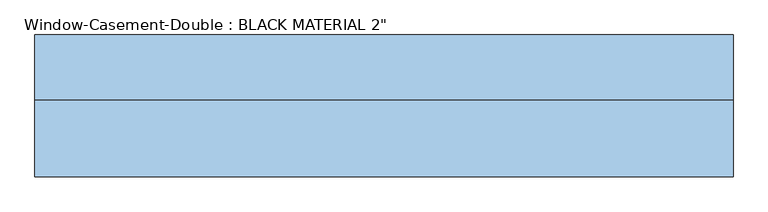
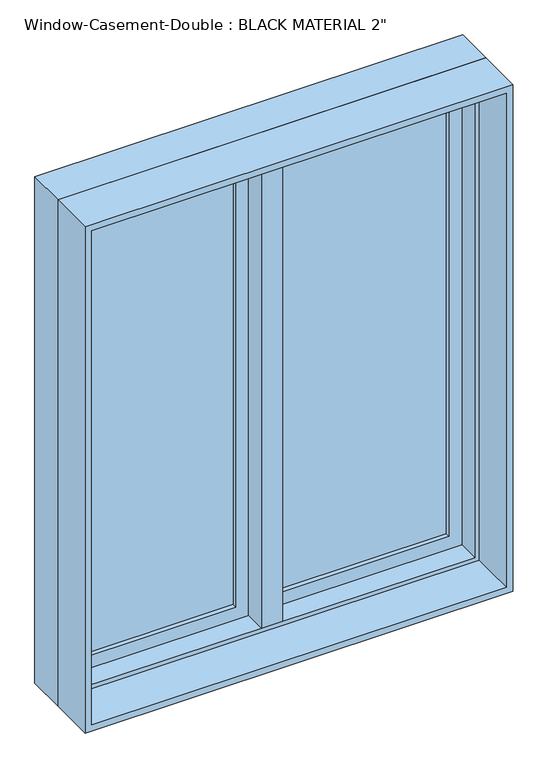
"""IFC4 building model written with IfcOpenShell, lengths in millimetres: window geometry."""

from ifc_helpers import new_model, si_unit, frame, origin, place, context, project, spatial, polyline, outline, extrude, faceted_brep, source, transform, mapped, element, save


def window_8377141f(model_context):
    return source(origin(), model_context, "Body", "SolidModel", [
        faceted_brep([(9.525, 133.35, 2425.7), (-9.525, 133.35, 2425.7), (-9.525, 82.55, 2425.7), (9.525, 82.55, 2425.7), (9.525, 133.35, 927.1), (9.525, 82.55, 927.1), (-9.525, 82.55, 927.1), (-9.525, 133.35, 927.1), (-9.525, 82.55, 946.15), (-9.525, 82.55, 2406.65), (-30.1625, 82.55, 946.15), (-30.1625, 82.55, 2406.65), (-30.1625, 19.05, 946.15), (-30.1625, 19.05, 2406.65), (30.1625, 19.05, 946.15), (30.1625, 19.05, 2406.65), (30.1625, 82.55, 946.15), (30.1625, 82.55, 2406.65), (9.525, 82.55, 946.15), (9.525, 82.55, 2406.65)], [[[0, 1, 2, 3]], [[4, 5, 6, 7]], [[1, 0, 4, 7]], [[2, 1, 7, 6, 8, 9]], [[9, 8, 10, 11]], [[11, 10, 12, 13]], [[13, 12, 14, 15]], [[15, 14, 16, 17]], [[17, 16, 18, 19]], [[0, 3, 19, 18, 5, 4]], [[18, 8, 6, 5]], [[9, 19, 3, 2]], [[8, 18, 16, 14, 12, 10]], [[19, 9, 11, 13, 15, 17]]]),
        extrude(outline(polyline([(-66.675, 114.3), (-66.675, 107.95), (-539.75, 107.95), (-539.75, 114.3), (-66.675, 114.3)])), frame((0.0, 0.0, 984.25), z_axis=(0.0, 0.0, 1.0), x_axis=(1.0, 0.0, 0.0)), (0.0, 0.0, 1.0), 1384.3),
        extrude(outline(polyline([(-539.75, 95.25), (-539.75, 101.6), (-66.675, 101.6), (-66.675, 95.25), (-539.75, 95.25)])), frame((0.0, 0.0, 984.25), z_axis=(0.0, 0.0, 1.0), x_axis=(1.0, 0.0, 0.0)), (0.0, 0.0, 1.0), 1384.3),
        extrude(outline(polyline([(539.75, 114.3), (539.75, 107.95), (66.675, 107.95), (66.675, 114.3), (539.75, 114.3)])), frame((0.0, 0.0, 984.25), z_axis=(0.0, 0.0, 1.0), x_axis=(1.0, 0.0, 0.0)), (0.0, 0.0, 1.0), 1384.3),
        extrude(outline(polyline([(66.675, 95.25), (66.675, 101.6), (539.75, 101.6), (539.75, 95.25), (66.675, 95.25)])), frame((0.0, 0.0, 984.25), z_axis=(0.0, 0.0, 1.0), x_axis=(1.0, 0.0, 0.0)), (0.0, 0.0, 1.0), 1384.3),
        extrude(outline(polyline([(2425.7, -596.9), (927.1, -596.9), (927.1, -9.525), (2425.7, -9.525), (2425.7, -596.9)]), holes=[polyline([(2368.55, -66.675), (984.25, -66.675), (984.25, -539.75), (2368.55, -539.75), (2368.55, -66.675)])]), frame((0.0, 82.55, 0.0), z_axis=(0.0, 1.0, 0.0), x_axis=(0.0, 0.0, 1.0)), (0.0, 0.0, 1.0), 44.45),
        extrude(outline(polyline([(927.1, 596.9), (2425.7, 596.9), (2425.7, 9.525), (927.1, 9.525), (927.1, 596.9)]), holes=[polyline([(984.25, 66.675), (2368.55, 66.675), (2368.55, 539.75), (984.25, 539.75), (984.25, 66.675)])]), frame((0.0, 82.55, 0.0), z_axis=(0.0, 1.0, 0.0), x_axis=(0.0, 0.0, 1.0)), (0.0, 0.0, 1.0), 44.45),
        extrude(outline(polyline([(2438.4, -609.6), (914.4, -609.6), (914.4, 609.6), (2438.4, 609.6), (2438.4, -609.6)]), holes=[polyline([(2419.35, 590.55), (933.45, 590.55), (933.45, -590.55), (2419.35, -590.55), (2419.35, 590.55)])]), frame((0.0, -114.3, 0.0), z_axis=(0.0, 1.0, 0.0), x_axis=(0.0, 0.0, 1.0)), (0.0, 0.0, 1.0), 133.35),
        faceted_brep([(577.85, 82.55, 2406.65), (577.85, 19.05, 2406.65), (-577.85, 19.05, 2406.65), (-577.85, 82.55, 2406.65), (596.9, 133.35, 2425.7), (596.9, 82.55, 2425.7), (-596.9, 82.55, 2425.7), (-596.9, 133.35, 2425.7), (609.6, 19.05, 2438.4), (609.6, 133.35, 2438.4), (-609.6, 133.35, 2438.4), (-609.6, 19.05, 2438.4), (-577.85, 19.05, 946.15), (-577.85, 82.55, 946.15), (-596.9, 82.55, 927.1), (-596.9, 133.35, 927.1), (-609.6, 133.35, 914.4), (-609.6, 19.05, 914.4), (577.85, 19.05, 946.15), (577.85, 82.55, 946.15), (596.9, 82.55, 927.1), (596.9, 133.35, 927.1), (609.6, 133.35, 914.4), (609.6, 19.05, 914.4)], [[[0, 1, 2, 3]], [[4, 5, 6, 7]], [[8, 9, 10, 11]], [[3, 2, 12, 13]], [[7, 6, 14, 15]], [[11, 10, 16, 17]], [[13, 12, 18, 19]], [[15, 14, 20, 21]], [[17, 16, 22, 23]], [[11, 17, 23, 8], [1, 18, 12, 2]], [[19, 18, 1, 0]], [[5, 20, 14, 6], [3, 13, 19, 0]], [[21, 20, 5, 4]], [[23, 22, 9, 8]], [[9, 22, 16, 10], [7, 15, 21, 4]]]),
    ])


if __name__ == "__main__":
    model = new_model("IFC4")
    model_context = context("Model", 3, world=origin())
    ifc_project = project(units=[si_unit("LENGTHUNIT", "METRE", prefix="MILLI")], contexts=[model_context])
    site = spatial("IfcSite", under=ifc_project)
    building = spatial("IfcBuilding", under=site)
    placement = place(None, origin())
    window_shape = window_8377141f(model_context)
    element("IfcWindow", 1, ObjectType="Window-Casement-Double : BLACK MATERIAL 2\"", at=placement, inside=building, context=model_context, shape_type="MappedRepresentation", body=[
        mapped(window_shape, transform((0.0, 0.0, 0.0), x_axis=(1.0, 0.0, 0.0), y_axis=(0.0, 1.0, 0.0), z_axis=(0.0, 0.0, 1.0))),
    ])
    save(model, "model.ifc")

# Revit data of these elements
# Type "Window-Casement-Double : BLACK MATERIAL 2\""
#   Type Mark = "18"
#   Fire Rating = "0.5h"
#   Assembly Code = "B2020100"
#   Analytic Construction = "Double glazing - domestic"
#   Frame Extension [instance default] = 0' - 0 1/4"
#   Window Inset [instance default] = 0' - 0"
#   Wall Thickness [instance default] = 0' - 6"
#   Interior Wall Closure [instance default] = 0' - 2 1/4"
#   Half Width = 2' - 0"
#   Visual Light Transmittance = 0.81
#   Thermal Resistance (R) = 1.8146 (h·ft²·°F)/BTU
#   Solar Heat Gain Coefficient = 0.76
#   Rough Width = 4' - 0 1/2"
#   Rough Height = 5' - 0 1/2"
#   Height = 5' - 0"
#   Heat Transfer Coefficient (U) = 0.5511 BTU/(h·ft²·°F)
#   Exterior Wall Closure [instance default] = 0' - 1 1/4"
#   Extension Jamb [instance default] = 0' - 2 1/4"
#   Default Sill Height = 3' - 0"
#   Width = 4' - 0"
#   Muntin Visibility = yes
#   Interior Trim Visibility [instance default] = yes
#   Exterior Trim Visibility [instance default] = yes
#   Extension Jamb Visibility [instance default] = yes
#   Interior Trim Material = Wood - Stained
#   Muntin Pattern = Muntin Pattern_2x2 : Muntin Pattern_2x2
#   Interior Trim = Trim-Window-Interior-Flat : Picture Frame
#   Interior Frame Material = Wood - Stained
#   Glass Panel Material = Glass
#   Exterior Trim Material = BLACK MATERIAL
#   Exterior Trim = Trim-Window-Exterior-Flat : with Sill
#   Exterior Frame Material = BLACK MATERIAL
#   Wall Closure = (empty or 0)
# Element 1 (IfcWindow, "Window-Casement-Double : BLACK MATERIAL 2\"")
#   Wall Thickness = 0' - 9"
#   Extension Jamb = 0' - 5 1/4"
#   Materials on its faces: "Wood - Stained", "Glass", "BLACK MATERIAL"
# Materials
#   "Wood - Stained": class "Wood", colour RGB 224 178 126, transparency 0, Cost = 0
#   "Glass": class "Glass", colour RGB 0 128 192, transparency 0.75, Description = "Soda Lime Glass", Cost = 0
#   "BLACK MATERIAL": class "Generic", colour RGB 120 120 120, transparency 0, Cost = 0
